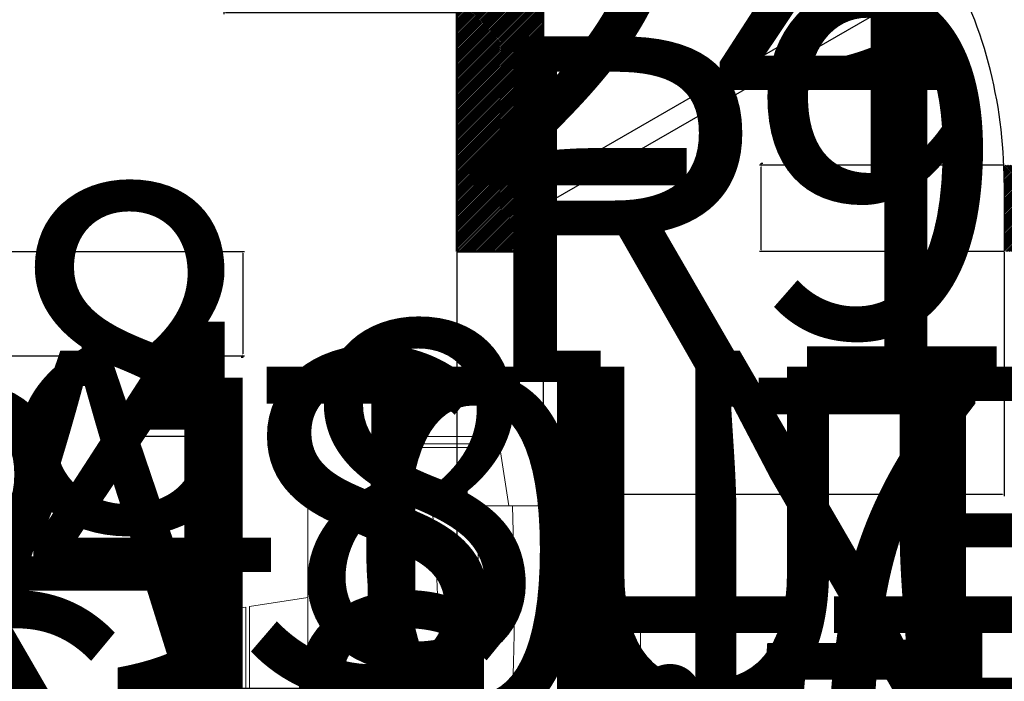
# Model space of a CAD drawing. Units: inches. Extents: x 1173 to 2157, y 515 to 1129.
# Tile 6 of 13: x 1475 to 1578, y 880 to 948. Entities that reach past the tile are written whole.
import ezdxf

# ---------------------------------------------------------------- set-up
doc = ezdxf.new("R2010")
doc.units = ezdxf.units.IN
doc.header["$MEASUREMENT"] = 0
for name, color, linetype, lineweight in [('A-ANNO-DIMS', 2, 'Continuous', 18), ('A-DOOR', 3, 'Continuous', 25), ('A-FURN', 8, 'Continuous', 18), ('A-WALL', 7, 'Continuous', 50)]:
    doc.layers.add(name, color=color, linetype=linetype, lineweight=lineweight)
doc.layers.add('A-WALL-PATT', color=22, linetype='Continuous', lineweight=13, true_color=0xca4b0c)
doc.styles.get("Standard").update_dxf_attribs({"font": 'arial.ttf'})
doc.dimstyles.get("Standard").update_dxf_attribs({"dimtxt": 36, "dimasz": 0.18, "dimexe": 0.18, "dimexo": 0.0625, "dimgap": 0.09, "dimtad": 0, "dimtih": 1, "dimtoh": 1, "dimdec": 0, "dimrnd": 72, "dimzin": 0, "dimdsep": 46, "dimlunit": 3, "dimtxsty": 'Standard', "dimcen": 2, "dimadec": 0, "dimazin": 0, "dimtfac": 1, "dimtdec": 0, "dimtofl": 0, "dimtmove": 0, "dimatfit": 3, "dimfxl": 1, "dimtolj": 1, "dimtzin": 0, "dimarcsym": 0})

# ---------------------------------------------------------------- blocks, each defined once
blk = doc.blocks.new('*U3')
for p, q in [((0, 0), (0, -6)), ((40, 0), (40, -6))]:
    blk.add_line(p, q)
blk.add_lwpolyline([(0, 0), (34.641, 20), (35.516, 18.484), (0.875, -1.516)], close=True)
blk.add_arc((0, 0), 40, 0, 30)
blk = doc.blocks.new('Dining Set - 36 x 72 in.')
for p, q in [((-22, 27.5), (-22.1562, 26.50042)), ((-22, 27.5), (-6, 27.5)), ((-5.8437, 26.49966), (-6, 27.5)), ((6, 27.5), (5.8438, 26.50042)), ((6, 27.5), (22, 27.5)), ((22.1563, 26.49966), (22, 27.5)), ((-22.2343, 26.00059), (-23.4847, 17.99762)), ((-22.2304, 26), (-5.7608, 26)), ((-5.8416, 26.5), (-22.1534, 26.5)), ((-4.5152, 17.99762), (-5.7655, 25.99926)), ((5.7657, 26.00059), (4.5153, 17.99762)), ((5.7696, 26), (22.2392, 26)), ((22.1584, 26.5), (5.8466, 26.5)), ((23.4848, 17.99762), (22.2345, 25.99926)), ((36, 18), (-36, 18)), ((-36, 18), (-36, -18)), ((36, -18), (36, 18)), ((-44.0006, 8.23428), (-35.9976, 9.48474)), ((44.0006, 8.23428), (35.9976, 9.48474)), ((-45.5, 8), (-44.5004, 8.15617)), ((-44.5, -8.15843), (-44.5, 8.15338)), ((-44, 8.23041), (-44, -8.23915)), ((44, 8.23041), (44, -8.23915)), ((44.5, -8.15843), (44.5, 8.15338)), ((45.5, 8), (44.5005, 8.15617)), ((-45.5, 8), (-45.5, -8)), ((45.5, 8), (45.5, -8)), ((-44.4997, -8.15631), (-45.5, -8)), ((44.4997, -8.15631), (45.5, -8)), ((-35.9976, -9.48476), (-43.9993, -8.2345)), ((35.9976, -9.48476), (43.9993, -8.2345)), ((-36, -18), (36, -18)), ((-22.2343, -26.0006), (-23.4847, -17.99762)), ((-4.5152, -17.99762), (-5.7655, -25.99928)), ((5.7657, -26.0006), (4.5153, -17.99762)), ((23.4848, -17.99762), (22.2345, -25.99928)), ((-22.2304, -26), (-5.7608, -26)), ((-22, -27.5), (-22.1562, -26.50044)), ((-5.8416, -26.5), (-22.1534, -26.5)), ((-5.8437, -26.49967), (-6, -27.5)), ((5.7696, -26), (22.2392, -26)), ((6, -27.5), (5.8438, -26.50044)), ((22.1584, -26.5), (5.8466, -26.5)), ((22.1563, -26.49967), (22, -27.5)), ((-22, -27.5), (-6, -27.5)), ((6, -27.5), (22, -27.5))]:
    blk.add_line(p, q)
for points in [[(-36, 15), (-31.1772, 14.97754), (-26.8079, 14.91406), (-22.8538, 14.81543), (-19.276, 14.6875), (-16.0362, 14.53613), (-13.0957, 14.36718), (-10.4159, 14.18652), (-7.9583, 14), (-5.6904, 13.81315), (-3.6035, 13.63021), (-1.6954, 13.45508), (0.0365, 13.29166), (1.5945, 13.14388), (2.9811, 13.01562), (4.1988, 12.9108), (5.25, 12.83333), (6.1393, 12.78613), (6.8802, 12.76823), (7.4883, 12.77767), (7.9792, 12.8125), (8.3685, 12.87077), (8.6719, 12.95052), (8.9049, 13.0498), (9.0833, 13.16666), (9.2205, 13.29899), (9.3216, 13.44401), (9.3895, 13.59879), (9.4271, 13.76041), (9.4373, 13.92594), (9.4232, 14.09245), (9.3875, 14.257), (9.3333, 14.41666), (9.2638, 14.56917), (9.1836, 14.71484), (9.0975, 14.85465), (9.0104, 14.98958), (8.9272, 15.1206), (8.8529, 15.2487), (8.7922, 15.37483), (8.75, 15.5), (8.7305, 15.62467), (8.7344, 15.74739), (8.7617, 15.86621), (8.8125, 15.97916), (8.8867, 16.08431), (8.9844, 16.17968), (9.1055, 16.26334), (9.25, 16.33333), (9.4189, 16.38802), (9.6172, 16.42708), (9.8506, 16.45052), (10.125, 16.45833), (10.4463, 16.45052), (10.8203, 16.42708), (11.2529, 16.38802), (11.75, 16.33333), (12.3184, 16.26318), (12.9694, 16.17838), (13.7151, 16.07991), (14.5677, 15.96875), (15.5395, 15.84586), (16.6426, 15.71224), (17.8893, 15.56884), (19.2917, 15.41666), (20.859, 15.25667), (22.5879, 15.08984), (24.4721, 14.91715), (26.5052, 14.73958), (28.6809, 14.5581), (30.9929, 14.3737), (33.4347, 14.18733), (36, 14)], [(-36, 10), (-28.9766, 10.14274), (-23.1725, 10.20442), (-18.4241, 10.19775), (-14.5677, 10.13541), (-11.4399, 10.03011), (-8.877, 9.89453), (-6.7154, 9.74137), (-4.7917, 9.58333), (-2.9698, 9.43082), (-1.2246, 9.28515), (0.4415, 9.14534), (2.026, 9.01041), (3.5266, 8.87939), (4.9408, 8.7513), (6.266, 8.62516), (7.5, 8.5), (8.6411, 8.37549), (9.6914, 8.2539), (10.6538, 8.13818), (11.5312, 8.03125), (12.3267, 7.93603), (13.043, 7.85547), (13.6831, 7.79248), (14.25, 7.75), (14.7471, 7.7303), (15.1797, 7.73307), (15.5537, 7.75732), (15.875, 7.80208), (16.1494, 7.86637), (16.3828, 7.94922), (16.5811, 8.04964), (16.75, 8.16666), (16.8944, 8.29915), (17.0143, 8.44531), (17.1089, 8.60319), (17.1771, 8.77083), (17.218, 8.94629), (17.2305, 9.1276), (17.2137, 9.31282), (17.1667, 9.5), (17.0895, 9.6875), (16.987, 9.875), (16.8649, 10.0625), (16.7292, 10.25), (16.5856, 10.4375), (16.4401, 10.625), (16.2985, 10.8125), (16.1667, 11), (16.05, 11.18733), (15.9518, 11.3737), (15.8752, 11.5581), (15.8229, 11.73958), (15.798, 11.91715), (15.8034, 12.08984), (15.842, 12.25667), (15.9167, 12.41666), (16.0295, 12.56836), (16.1784, 12.70833), (16.3605, 12.83268), (16.5729, 12.9375), (16.8127, 13.01888), (17.0768, 13.07291), (17.3625, 13.0957), (17.6667, 13.08333), (17.9894, 13.03312), (18.3418, 12.94726), (18.7382, 12.82918), (19.1927, 12.68229), (19.7195, 12.51001), (20.3327, 12.31575), (21.0465, 12.10294), (21.875, 11.875), (22.8357, 11.63354), (23.959, 11.37304), (25.2786, 11.08618), (26.8282, 10.76562), (28.6414, 10.40405), (30.752, 9.99414), (33.1936, 9.52856), (36, 9)], [(-36, 5.5), (-30.7157, 5.3348), (-26.069, 5.20963), (-21.9946, 5.11767), (-18.4271, 5.05208), (-15.3009, 5.00602), (-12.5508, 4.97265), (-10.1112, 4.94515), (-7.9167, 4.91666), (-5.909, 4.88167), (-4.0586, 4.83984), (-2.3429, 4.79215), (-0.7396, 4.73958), (0.7739, 4.6831), (2.22, 4.6237), (3.6213, 4.56233), (5, 4.5), (6.373, 4.43782), (7.7344, 4.3776), (9.0723, 4.32129), (10.375, 4.27083), (11.6309, 4.22819), (12.8281, 4.19531), (13.9551, 4.17415), (15, 4.16666), (15.954, 4.17448), (16.819, 4.19791), (17.6001, 4.23698), (18.3021, 4.29166), (18.9299, 4.36198), (19.4883, 4.44791), (19.9823, 4.54948), (20.4167, 4.66666), (20.7969, 4.79899), (21.1302, 4.94401), (21.4245, 5.09879), (21.6875, 5.26041), (21.9271, 5.42594), (22.1511, 5.59245), (22.3672, 5.757), (22.5834, 5.91666), (22.8065, 6.06868), (23.0404, 6.21093), (23.2879, 6.34147), (23.5521, 6.45833), (23.8358, 6.55957), (24.142, 6.64323), (24.4735, 6.70735), (24.8334, 6.75), (25.2235, 6.76969), (25.642, 6.76692), (26.0858, 6.74267), (26.5521, 6.69791), (27.0379, 6.63362), (27.5404, 6.55078), (28.0565, 6.45036), (28.5834, 6.33333), (29.1242, 6.19987), (29.7071, 6.04687), (30.3661, 5.87044), (31.1354, 5.66666), (32.0493, 5.43164), (33.142, 5.16146), (34.4475, 4.85221), (36, 4.5)], [(-36, -1), (-30.7915, -0.6591), (-26.0195, -0.38216), (-21.6519, -0.16284), (-17.6563, 0.00521), (-14.0005, 0.12833), (-10.6523, 0.21289), (-7.5796, 0.26522), (-4.75, 0.29166), (-2.134, 0.29793), (0.2878, 0.28711), (2.5317, 0.26163), (4.6146, 0.22396), (6.5529, 0.17651), (8.3633, 0.12174), (10.0623, 0.06209), (11.6667, 0), (13.1899, -0.06201), (14.6341, -0.1211), (15.9982, -0.17432), (17.2813, -0.21875), (18.4823, -0.25147), (19.6003, -0.26953), (20.6343, -0.27002), (21.5834, -0.25), (22.4481, -0.20768), (23.2357, -0.14584), (23.9549, -0.06836), (24.6146, 0.02083), (25.2235, 0.11784), (25.7904, 0.21875), (26.3241, 0.31966), (26.8334, 0.41666), (27.3265, 0.50618), (27.8099, 0.58593), (28.2894, 0.65397), (28.7709, 0.70833), (29.2601, 0.74707), (29.763, 0.76823), (30.2855, 0.76985), (30.8334, 0.75), (31.4088, 0.70784), (31.9994, 0.64713), (32.589, 0.57275), (33.1615, 0.48958), (33.7008, 0.4025), (34.1908, 0.3164), (34.6153, 0.23616), (34.9584, 0.16666), (35.2099, 0.11165), (35.3848, 0.07031), (35.504, 0.04069), (35.5886, 0.02083), (35.6594, 0.00879), (35.7377, 0.0026), (35.8442, 0.00032), (36, 0)], [(-36, -6.5), (-27.1843, -6.31267), (-20.084, -6.1263), (-14.469, -5.9419), (-10.1094, -5.76042), (-6.7752, -5.58285), (-4.2363, -5.41016), (-2.2629, -5.24333), (-0.625, -5.08334), (0.8708, -4.93099), (2.2715, -4.78646), (3.5872, -4.64974), (4.8281, -4.52084), (6.0046, -4.39974), (7.127, -4.28646), (8.2053, -4.18099), (9.25, -4.08334), (10.2705, -3.99382), (11.2734, -3.91407), (12.2647, -3.84603), (13.25, -3.79167), (14.2354, -3.75293), (15.2266, -3.73177), (16.2295, -3.73015), (17.25, -3.75), (18.2912, -3.79248), (19.3451, -3.85547), (20.4009, -3.93604), (21.4479, -4.03125), (22.4754, -4.13819), (23.4727, -4.25391), (24.4289, -4.37549), (25.3334, -4.5), (26.1785, -4.62492), (26.9694, -4.74935), (27.7145, -4.87281), (28.4219, -4.99479), (29.1, -5.11483), (29.7572, -5.23242), (30.4016, -5.34709), (31.0417, -5.45834), (31.6837, -5.56437), (32.3262, -5.65821), (32.9658, -5.73153), (33.599, -5.77604), (34.2224, -5.78345), (34.8327, -5.74545), (35.4264, -5.65373), (36, -5.5)], [(-36, -10), (-26.4022, -9.81299), (-18.4675, -9.62891), (-11.9839, -9.45069), (-6.7396, -9.28125), (-2.5226, -9.12354), (0.8789, -8.98047), (3.6769, -8.85498), (6.0833, -8.75), (8.2767, -8.66765), (10.3021, -8.60677), (12.1712, -8.56543), (13.8958, -8.54167), (15.4876, -8.53353), (16.9583, -8.53907), (18.3197, -8.55632), (19.5834, -8.58334), (20.7616, -8.61841), (21.8685, -8.66081), (22.9188, -8.71004), (23.9271, -8.76563), (24.9081, -8.82707), (25.8763, -8.89388), (26.8465, -8.96558), (27.8334, -9.04167), (28.8474, -9.12118), (29.8828, -9.20117), (30.93, -9.27824), (31.9792, -9.34896), (33.0205, -9.40991), (34.0443, -9.45768), (35.0407, -9.48885), (36, -9.5)], [(-36, -14.5), (-30.0881, -14.33513), (-25.0332, -14.21224), (-20.7312, -14.12647), (-17.0781, -14.07292), (-13.97, -14.04671), (-11.3027, -14.04297), (-8.9724, -14.05681), (-6.875, -14.08334), (-4.9224, -14.11833), (-3.0905, -14.16016), (-1.3709, -14.20785), (0.2448, -14.26042), (1.7647, -14.3169), (3.1973, -14.3763), (4.5507, -14.43767), (5.8333, -14.5), (7.0554, -14.5621), (8.235, -14.62175), (9.3922, -14.67652), (10.5469, -14.72396), (11.7192, -14.76164), (12.929, -14.78711), (14.1965, -14.79794), (15.5417, -14.79167), (16.9933, -14.76424), (18.6152, -14.70508), (20.4804, -14.60197), (22.6615, -14.44271), (25.2312, -14.21509), (28.2624, -13.9069), (31.8277, -13.50594), (36, -13)]]:
    blk.add_lwpolyline(points)
blk = doc.blocks.new('*D36')
at = {"layer": 'A-ANNO-DIMS', "color": 0, "lineweight": -2, "transparency": 16777216}
for p, q in [((1497.87, 905.02), (1487.37, 905.02)), ((1487.55, 904.84), (1487.55, 889.09)), ((1487.55, 835.93), (1487.55, 851.68)), ((1497.87, 835.75), (1487.37, 835.75))]:
    blk.add_line(p, q, dxfattribs=at)
at = {"layer": 'A-ANNO-DIMS', "color": 0, "transparency": 16777216}
for points in [[(1487.52, 904.84), (1487.58, 904.84), (1487.55, 905.02)], [(1487.52, 835.93), (1487.58, 835.93), (1487.55, 835.75)]]:
    blk.add_solid(points, dxfattribs=at)
at = {"layer": 'Defpoints', "color": 0, "transparency": 16777216}
for p in [(1497.94, 905.02), (1487.55, 835.75), (1497.94, 835.75)]:
    blk.add_point(p, dxfattribs=at)
at = {"layer": 'A-ANNO-DIMS', "color": 0, "transparency": 16777216, "insert": (1487.55, 870.38), "char_height": 36, "attachment_point": 5}
blk.add_mtext('\\A1;DINING SET 69', dxfattribs=at)
blk = doc.blocks.new('*D38')
at = {"layer": 'A-ANNO-DIMS', "color": 0, "lineweight": -2, "transparency": 16777216}
for p, q in [((1471.69, 862.7), (1478.04, 862.7)), ((1477.86, 862.52), (1477.86, 860.65)), ((1477.86, 821.35), (1477.86, 823.22)), ((1471.69, 821.17), (1478.04, 821.17))]:
    blk.add_line(p, q, dxfattribs=at)
at = {"layer": 'A-ANNO-DIMS', "color": 0, "transparency": 16777216}
for points in [[(1477.83, 862.52), (1477.89, 862.52), (1477.86, 862.7)], [(1477.83, 821.35), (1477.89, 821.35), (1477.86, 821.17)]]:
    blk.add_solid(points, dxfattribs=at)
at = {"layer": 'Defpoints', "color": 0, "transparency": 16777216}
for p in [(1471.63, 862.7), (1477.86, 862.7), (1471.63, 821.17)]:
    blk.add_point(p, dxfattribs=at)
at = {"layer": 'A-ANNO-DIMS', "color": 0, "transparency": 16777216, "insert": (1477.86, 841.93), "char_height": 36, "attachment_point": 5}
blk.add_mtext('\\A1;COFFEE TABLE 42', dxfattribs=at)
blk = doc.blocks.new('*D40')
at = {"layer": 'A-ANNO-DIMS', "color": 0, "lineweight": -2, "transparency": 16777216}
for p, q in [((1422.73, 872.86), (1431.84, 872.86)), ((1431.66, 872.68), (1431.66, 861.58)), ((1431.66, 813.04), (1431.66, 824.15)), ((1422.73, 812.86), (1431.84, 812.86))]:
    blk.add_line(p, q, dxfattribs=at)
at = {"layer": 'A-ANNO-DIMS', "color": 0, "transparency": 16777216}
for points in [[(1431.63, 872.68), (1431.69, 872.68), (1431.66, 872.86)], [(1431.63, 813.04), (1431.69, 813.04), (1431.66, 812.86)]]:
    blk.add_solid(points, dxfattribs=at)
at = {"layer": 'Defpoints', "color": 0, "transparency": 16777216}
for p in [(1422.66, 872.86), (1431.66, 872.86), (1422.66, 812.86)]:
    blk.add_point(p, dxfattribs=at)
at = {"layer": 'A-ANNO-DIMS', "color": 0, "transparency": 16777216, "insert": (1431.66, 842.86), "char_height": 36, "attachment_point": 5}
blk.add_mtext('\\A1;LOVESEAT 60', dxfattribs=at)
blk = doc.blocks.new('*D46')
at = {"layer": 'A-ANNO-DIMS', "color": 0, "lineweight": -2, "transparency": 16777216}
for p, q in [((1646.37, 911.98), (1645.86, 896.32)), ((1648.72, 912.09), (1646.2, 912.17)), ((1645.85, 895.96), (1645.67, 895.96)), ((1648.2, 896.07), (1645.68, 896.15)), ((1645.86, 896.14), (1645.85, 895.96))]:
    blk.add_line(p, q, dxfattribs=at)
at = {"layer": 'A-ANNO-DIMS', "color": 0, "transparency": 16777216}
for points in [[(1646.34, 911.99), (1646.4, 911.98), (1646.38, 912.16)], [(1645.83, 896.32), (1645.89, 896.32), (1645.86, 896.14)]]:
    blk.add_solid(points, dxfattribs=at)
at = {"layer": 'Defpoints', "color": 0, "transparency": 16777216}
for p in [(1648.78, 912.09), (1645.86, 896.14), (1648.26, 896.06)]:
    blk.add_point(p, dxfattribs=at)
at = {"layer": 'A-ANNO-DIMS', "color": 0, "transparency": 16777216, "insert": (1538.16, 895.96), "char_height": 36, "attachment_point": 5}
blk.add_mtext('\\A1;BASIN 16', dxfattribs=at)
blk = doc.blocks.new('*D48')
at = {"layer": 'A-ANNO-DIMS', "color": 0, "lineweight": -2, "transparency": 16777216}
for p, q in [((1592.53, 826.46), (1592.35, 826.47)), ((1592.38, 821.85), (1592.54, 826.64)), ((1623.53, 825.46), (1592.71, 826.46)), ((1623.56, 820.84), (1623.71, 825.64))]:
    blk.add_line(p, q, dxfattribs=at)
at = {"layer": 'A-ANNO-DIMS', "color": 0, "transparency": 16777216}
for points in [[(1592.71, 826.49), (1592.71, 826.43), (1592.53, 826.46)], [(1623.53, 825.49), (1623.53, 825.43), (1623.71, 825.46)]]:
    blk.add_solid(points, dxfattribs=at)
at = {"layer": 'Defpoints', "color": 0, "transparency": 16777216}
for p in [(1592.53, 826.46), (1592.38, 821.79), (1623.56, 820.78)]:
    blk.add_point(p, dxfattribs=at)
at = {"layer": 'A-ANNO-DIMS', "color": 0, "transparency": 16777216, "insert": (1488.3, 826.47), "char_height": 36, "attachment_point": 5}
blk.add_mtext('\\A1;BASIN 31', dxfattribs=at)
blk = doc.blocks.new('*D50')
at = {"layer": 'A-ANNO-DIMS', "color": 0, "lineweight": -2, "transparency": 16777216}
for p, q in [((1603.33, 798.21), (1603.33, 796.59)), ((1613.33, 798.21), (1613.33, 796.59)), ((1603.33, 796.77), (1603.15, 796.77)), ((1613.15, 796.77), (1603.51, 796.77))]:
    blk.add_line(p, q, dxfattribs=at)
at = {"layer": 'A-ANNO-DIMS', "color": 0, "transparency": 16777216}
for points in [[(1603.51, 796.8), (1603.51, 796.74), (1603.33, 796.77)], [(1613.15, 796.8), (1613.15, 796.74), (1613.33, 796.77)]]:
    blk.add_solid(points, dxfattribs=at)
at = {"layer": 'Defpoints', "color": 0, "transparency": 16777216}
for p in [(1603.33, 798.27), (1613.33, 798.27), (1603.33, 796.77)]:
    blk.add_point(p, dxfattribs=at)
at = {"layer": 'A-ANNO-DIMS', "color": 0, "transparency": 16777216, "insert": (1377.9, 796.77), "char_height": 36, "attachment_point": 5}
blk.add_mtext('\\A1;BASIN TAP 10 TYP.', dxfattribs=at)
blk = doc.blocks.new('*D52')
at = {"layer": 'A-ANNO-DIMS', "color": 0, "lineweight": -2, "transparency": 16777216}
for p, q in [((1589.6, 924.28), (1580.48, 924.28)), ((1580.66, 924.1), (1580.66, 912.75)), ((1580.66, 864.46), (1580.66, 875.81)), ((1589.6, 864.28), (1580.48, 864.28))]:
    blk.add_line(p, q, dxfattribs=at)
at = {"layer": 'A-ANNO-DIMS', "color": 0, "transparency": 16777216}
for points in [[(1580.63, 924.1), (1580.69, 924.1), (1580.66, 924.28)], [(1580.63, 864.46), (1580.69, 864.46), (1580.66, 864.28)]]:
    blk.add_solid(points, dxfattribs=at)
at = {"layer": 'Defpoints', "color": 0, "transparency": 16777216}
for p in [(1580.66, 924.28), (1589.66, 924.28), (1589.66, 864.28)]:
    blk.add_point(p, dxfattribs=at)
at = {"layer": 'A-ANNO-DIMS', "color": 0, "transparency": 16777216, "insert": (1580.66, 894.28), "char_height": 36, "attachment_point": 5}
blk.add_mtext('\\A1;TUB 60', dxfattribs=at)
blk = doc.blocks.new('*D54')
at = {"layer": 'A-ANNO-DIMS', "color": 0, "lineweight": -2, "transparency": 16777216}
for p, q in [((1496.35, 1005.18), (1488.93, 1005.18)), ((1489.11, 1005), (1489.11, 999.54)), ((1489.11, 956.65), (1489.11, 962.11)), ((1496.35, 956.47), (1488.93, 956.47))]:
    blk.add_line(p, q, dxfattribs=at)
at = {"layer": 'A-ANNO-DIMS', "color": 0, "transparency": 16777216}
for points in [[(1489.08, 1005), (1489.14, 1005), (1489.11, 1005.18)], [(1489.08, 956.65), (1489.14, 956.65), (1489.11, 956.47)]]:
    blk.add_solid(points, dxfattribs=at)
at = {"layer": 'Defpoints', "color": 0, "transparency": 16777216}
for p in [(1496.42, 1005.18), (1489.11, 956.47), (1496.42, 956.47)]:
    blk.add_point(p, dxfattribs=at)
at = {"layer": 'A-ANNO-DIMS', "color": 0, "transparency": 16777216, "insert": (1489.11, 980.83), "char_height": 36, "attachment_point": 5}
blk.add_mtext('\\A1;WORK TABLE 49', dxfattribs=at)
blk = doc.blocks.new('*D55')
at = {"layer": 'A-ANNO-DIMS', "color": 0, "lineweight": -2, "transparency": 16777216}
for p, q in [((1496.42, 956.41), (1496.42, 948.98)), ((1520.77, 956.41), (1520.77, 948.98)), ((1496.6, 949.16), (1520.59, 949.16)), ((1520.77, 949.16), (1520.95, 949.16))]:
    blk.add_line(p, q, dxfattribs=at)
at = {"layer": 'A-ANNO-DIMS', "color": 0, "transparency": 16777216}
for points in [[(1496.6, 949.19), (1496.6, 949.13), (1496.42, 949.16)], [(1520.59, 949.19), (1520.59, 949.13), (1520.77, 949.16)]]:
    blk.add_solid(points, dxfattribs=at)
at = {"layer": 'Defpoints', "color": 0, "transparency": 16777216}
for p in [(1496.42, 956.47), (1520.77, 956.47), (1520.77, 949.16)]:
    blk.add_point(p, dxfattribs=at)
at = {"layer": 'A-ANNO-DIMS', "color": 0, "transparency": 16777216, "insert": (1547.06, 949.16), "char_height": 36, "attachment_point": 5}
blk.add_mtext('\\A1;24', dxfattribs=at)
blk = doc.blocks.new('*D56')
at = {"layer": 'A-ANNO-DIMS', "color": 0, "lineweight": -2, "transparency": 16777216}
for p, q in [((1426.92, 1014.79), (1433.2, 1014.79)), ((1433.02, 1014.61), (1433.02, 1012.98)), ((1433.02, 973.94), (1433.02, 975.57)), ((1426.92, 973.76), (1433.2, 973.76))]:
    blk.add_line(p, q, dxfattribs=at)
at = {"layer": 'A-ANNO-DIMS', "color": 0, "transparency": 16777216}
for points in [[(1432.99, 1014.61), (1433.05, 1014.61), (1433.02, 1014.79)], [(1432.99, 973.94), (1433.05, 973.94), (1433.02, 973.76)]]:
    blk.add_solid(points, dxfattribs=at)
at = {"layer": 'Defpoints', "color": 0, "transparency": 16777216}
for p in [(1426.86, 1014.79), (1433.02, 1014.79), (1426.86, 973.76)]:
    blk.add_point(p, dxfattribs=at)
at = {"layer": 'A-ANNO-DIMS', "color": 0, "transparency": 16777216, "insert": (1433.02, 994.27), "char_height": 36, "attachment_point": 5}
blk.add_mtext('\\A1;RANGE 41', dxfattribs=at)
blk = doc.blocks.new('*D60')
at = {"layer": 'A-ANNO-DIMS', "color": 0, "lineweight": -2, "transparency": 16777216}
for p, q in [((1390.73, 971.62), (1390.73, 971.8)), ((1390.73, 971.8), (1390.91, 971.8)), ((1396.06, 971.62), (1390.55, 971.62)), ((1390.73, 935.8), (1390.73, 971.44)), ((1396.06, 935.62), (1390.55, 935.62))]:
    blk.add_line(p, q, dxfattribs=at)
at = {"layer": 'A-ANNO-DIMS', "color": 0, "transparency": 16777216}
for points in [[(1390.7, 971.44), (1390.76, 971.44), (1390.73, 971.62)], [(1390.7, 935.8), (1390.76, 935.8), (1390.73, 935.62)]]:
    blk.add_solid(points, dxfattribs=at)
at = {"layer": 'Defpoints', "color": 0, "transparency": 16777216}
for p in [(1390.73, 971.62), (1396.13, 971.62), (1396.13, 935.62)]:
    blk.add_point(p, dxfattribs=at)
at = {"layer": 'A-ANNO-DIMS', "color": 0, "transparency": 16777216, "insert": (1517.73, 971.8), "char_height": 36, "attachment_point": 5}
blk.add_mtext('\\A1;FRIDGE 36', dxfattribs=at)
blk = doc.blocks.new('*D69')
at = {"layer": 'A-ANNO-DIMS', "color": 0, "lineweight": -2, "transparency": 16777216}
for p, q in [((1472.66, 924.22), (1472.66, 538.8)), ((1520.66, 924.22), (1520.66, 538.8)), ((1472.84, 538.98), (1520.48, 538.98)), ((1520.66, 538.98), (1520.84, 538.98))]:
    blk.add_line(p, q, dxfattribs=at)
at = {"layer": 'A-ANNO-DIMS', "color": 0, "transparency": 16777216}
for points in [[(1472.84, 539.01), (1472.84, 538.95), (1472.66, 538.98)], [(1520.48, 539.01), (1520.48, 538.95), (1520.66, 538.98)]]:
    blk.add_solid(points, dxfattribs=at)
at = {"layer": 'Defpoints', "color": 0, "transparency": 16777216}
for p in [(1472.66, 924.28), (1520.66, 924.28), (1520.66, 538.98)]:
    blk.add_point(p, dxfattribs=at)
at = {"layer": 'A-ANNO-DIMS', "color": 0, "transparency": 16777216, "insert": (1547.48, 538.98), "char_height": 36, "attachment_point": 5}
blk.add_mtext('\\A1;48', dxfattribs=at)
blk = doc.blocks.new('*D87')
at = {"layer": 'A-ANNO-DIMS', "color": 0, "lineweight": -2, "transparency": 16777216}
for p, q in [((1529.66, 924.22), (1529.66, 898.8)), ((1577.66, 924.22), (1577.66, 898.8)), ((1529.66, 898.98), (1529.48, 898.98)), ((1577.48, 898.98), (1529.84, 898.98))]:
    blk.add_line(p, q, dxfattribs=at)
at = {"layer": 'A-ANNO-DIMS', "color": 0, "transparency": 16777216}
for points in [[(1529.84, 899.01), (1529.84, 898.95), (1529.66, 898.98)], [(1577.48, 899.01), (1577.48, 898.95), (1577.66, 898.98)]]:
    blk.add_solid(points, dxfattribs=at)
at = {"layer": 'Defpoints', "color": 0, "transparency": 16777216}
for p in [(1529.66, 924.28), (1577.66, 924.28), (1529.66, 898.98)]:
    blk.add_point(p, dxfattribs=at)
at = {"layer": 'A-ANNO-DIMS', "color": 0, "transparency": 16777216, "insert": (1502.85, 898.98), "char_height": 36, "attachment_point": 5}
blk.add_mtext('\\A1;48', dxfattribs=at)
blk = doc.blocks.new('*D93')
at = {"layer": 'A-ANNO-DIMS', "color": 0, "lineweight": -2, "transparency": 16777216}
for p, q in [((1473.15, 924.28), (1498.57, 924.28)), ((1498.39, 924.1), (1498.39, 913.61)), ((1473.15, 913.43), (1498.57, 913.43)), ((1498.39, 913.25), (1498.21, 913.25)), ((1498.39, 913.43), (1498.39, 913.25))]:
    blk.add_line(p, q, dxfattribs=at)
at = {"layer": 'A-ANNO-DIMS', "color": 0, "transparency": 16777216}
for points in [[(1498.36, 924.1), (1498.42, 924.1), (1498.39, 924.28)], [(1498.36, 913.61), (1498.42, 913.61), (1498.39, 913.43)]]:
    blk.add_solid(points, dxfattribs=at)
at = {"layer": 'Defpoints', "color": 0, "transparency": 16777216}
for p in [(1473.08, 924.28), (1473.08, 913.43), (1498.39, 913.43)]:
    blk.add_point(p, dxfattribs=at)
at = {"layer": 'A-ANNO-DIMS', "color": 0, "transparency": 16777216, "insert": (1425.05, 913.25), "char_height": 36, "attachment_point": 5}
blk.add_mtext('\\A1;10.848', dxfattribs=at)
blk = doc.blocks.new('*D94')
at = {"layer": 'A-ANNO-DIMS', "color": 0, "lineweight": -2, "transparency": 16777216}
for p, q in [((1577.6, 933.28), (1552.18, 933.28)), ((1552.36, 933.28), (1552.36, 933.46)), ((1552.36, 933.46), (1552.54, 933.46)), ((1552.36, 924.46), (1552.36, 933.1)), ((1577.6, 924.28), (1552.18, 924.28))]:
    blk.add_line(p, q, dxfattribs=at)
at = {"layer": 'A-ANNO-DIMS', "color": 0, "transparency": 16777216}
for points in [[(1552.33, 933.1), (1552.39, 933.1), (1552.36, 933.28)], [(1552.33, 924.46), (1552.39, 924.46), (1552.36, 924.28)]]:
    blk.add_solid(points, dxfattribs=at)
at = {"layer": 'Defpoints', "color": 0, "transparency": 16777216}
for p in [(1552.36, 933.28), (1577.66, 933.28), (1577.66, 924.28)]:
    blk.add_point(p, dxfattribs=at)
at = {"layer": 'A-ANNO-DIMS', "color": 0, "transparency": 16777216, "insert": (1564.47, 933.46), "char_height": 36, "attachment_point": 5}
blk.add_mtext('\\A1;9', dxfattribs=at)
blk = doc.blocks.new('*D107')
at = {"layer": 'A-ANNO-DIMS', "color": 0, "lineweight": -2, "transparency": 16777216}
for p, q in [((1607.48, 928.68), (1607.66, 928.68)), ((1607.66, 928.68), (1607.66, 920.46)), ((1607.66, 904.28), (1607.66, 908.28)), ((1605.66, 906.28), (1609.66, 906.28))]:
    blk.add_line(p, q, dxfattribs=at)
at = {"layer": 'A-ANNO-DIMS', "color": 0, "transparency": 16777216}
blk.add_solid([(1607.69, 920.46), (1607.63, 920.46), (1607.66, 920.28)], dxfattribs=at)
at = {"layer": 'Defpoints', "color": 0, "transparency": 16777216}
for p in [(1607.66, 920.28), (1607.66, 906.28)]:
    blk.add_point(p, dxfattribs=at)
at = {"layer": 'A-ANNO-DIMS', "color": 0, "transparency": 16777216, "insert": (1564.46, 928.68), "char_height": 36, "attachment_point": 5}
blk.add_mtext('\\A1;R14', dxfattribs=at)
blk = doc.blocks.new('*D108')
at = {"layer": 'A-ANNO-DIMS', "color": 0, "lineweight": -2, "transparency": 16777216}
for p, q in [((1641.43, 881.4), (1641.43, 885.4)), ((1639.43, 883.4), (1643.43, 883.4)), ((1636.72, 865.51), (1638.44, 872.04)), ((1636.54, 865.51), (1636.72, 865.51))]:
    blk.add_line(p, q, dxfattribs=at)
at = {"layer": 'A-ANNO-DIMS', "color": 0, "transparency": 16777216}
blk.add_solid([(1638.41, 872.05), (1638.47, 872.04), (1638.49, 872.22)], dxfattribs=at)
at = {"layer": 'Defpoints', "color": 0, "transparency": 16777216}
for p in [(1641.43, 883.4), (1638.49, 872.22)]:
    blk.add_point(p, dxfattribs=at)
at = {"layer": 'A-ANNO-DIMS', "color": 0, "transparency": 16777216, "insert": (1505.59, 865.51), "char_height": 36, "attachment_point": 5}
blk.add_mtext('\\A1;2X R11.564', dxfattribs=at)
blk = doc.blocks.new('*D109')
at = {"layer": 'A-ANNO-DIMS', "color": 0, "lineweight": -2, "transparency": 16777216}
for p, q in [((1638.72, 893.14), (1638.9, 893.14)), ((1638.9, 893.14), (1639.74, 886.91)), ((1641.2, 874.07), (1641.2, 878.07)), ((1639.2, 876.07), (1643.2, 876.07))]:
    blk.add_line(p, q, dxfattribs=at)
at = {"layer": 'A-ANNO-DIMS', "color": 0, "transparency": 16777216}
blk.add_solid([(1639.77, 886.92), (1639.71, 886.91), (1639.77, 886.74)], dxfattribs=at)
at = {"layer": 'Defpoints', "color": 0, "transparency": 16777216}
for p in [(1639.77, 886.74), (1641.2, 876.07)]:
    blk.add_point(p, dxfattribs=at)
at = {"layer": 'A-ANNO-DIMS', "color": 0, "transparency": 16777216, "insert": (1507.71, 893.14), "char_height": 36, "attachment_point": 5}
blk.add_mtext('\\A1;2X R10.766', dxfattribs=at)

msp = doc.modelspace()

# ---------------------------------------------------------------- hatches: boundary and pattern name
at = {"layer": 'A-WALL-PATT'}
h = msp.add_hatch(dxfattribs=at)
h.set_pattern_fill('ANSI31', color=256)
h.paths.add_polyline_path([(1388.6635, 933.2805), (1388.6635, 1044.2805), (1413.7618, 1044.2805), (1413.7618, 1053.2805), (1379.6635, 1053.2805), (1379.6635, 894.1606), (1388.6635, 894.1606), (1388.6635, 924.2805), (1472.6635, 924.2805), (1472.6635, 933.2805)])
h.paths.add_polyline_path([(1520.6635, 1044.2805), (1520.6635, 1014.7866), (1520.6635, 1005.1794), (1520.7714, 1005.1794), (1520.7714, 956.4707), (1520.6635, 924.2805), (1529.6635, 924.2805), (1529.6635, 931.4788), (1529.6635, 1044.2805), (1530.8474, 1044.2805), (1570.9543, 1044.2805), (1570.9543, 1053.2805), (1461.7618, 1053.2805), (1461.7618, 1044.2805)])
h.paths.add_polyline_path([(1618.9543, 1053.2805), (1618.9543, 1044.2805), (1661.6635, 1044.2805), (1661.6635, 1043.7367), (1661.6635, 1032.8874), (1670.6635, 1032.8874), (1670.6635, 1053.2805)])
h.paths.add_polyline_path([(1661.6635, 933.2805), (1661.6635, 927.8377), (1661.6635, 924.2805), (1661.6635, 918.9156), (1670.6635, 918.9156), (1670.6635, 984.8874), (1661.6635, 984.8874), (1661.6635, 978.3712)])
h.paths.add_polyline_path([(1670.6635, 894.9156), (1661.6635, 894.9156), (1661.6635, 890.0349), (1661.9328, 890.0349), (1661.9328, 870.079), (1661.6635, 864.2805), (1589.6635, 864.2805), (1589.6635, 924.2805), (1625.553, 924.2805, -0.02455299), (1625.3782, 927.8377), (1625.3782, 933.2805), (1577.6635, 933.2805), (1577.6635, 924.2805), (1580.6635, 924.2805), (1580.6635, 855.2805), (1586.1062, 855.2805), (1589.6635, 855.2805), (1661.6635, 855.2805), (1661.6635, 826.5597), (1670.6635, 826.5597)])
h.paths.add_polyline_path([(1670.6635, 802.5597), (1661.6635, 802.5597), (1661.6635, 795.2805), (1589.6635, 795.2805), (1589.6635, 819.17, -0.02455299), (1586.1062, 818.9952), (1580.6635, 818.9952), (1580.6635, 795.2805), (1577.6635, 795.2805), (1577.6635, 786.2805), (1661.6635, 786.2805), (1661.6635, 778.5597), (1661.6635, 742.6973), (1670.6635, 742.6973)])
h.paths.add_polyline_path([(1661.6635, 654.2805), (1625.1498, 654.2805), (1625.1498, 645.2805), (1661.3656, 645.2805), (1661.6635, 645.2805), (1661.6635, 573.2805), (1520.6635, 573.2805), (1520.6635, 564.2805), (1670.6635, 564.2805), (1670.6635, 694.6973), (1661.6635, 694.6973)])
h.paths.add_polyline_path([(1529.4367, 733.4702, -0.06854064), (1529.6635, 734.2623), (1529.6635, 795.2805), (1520.6635, 795.2805), (1520.6635, 645.2805), (1577.1498, 645.2805), (1577.1498, 654.2805), (1529.6635, 654.2805), (1529.6635, 686.5626, -0.06854064), (1529.4367, 687.3547)])
h.paths.add_polyline_path([(1379.6635, 711.2805), (1388.6635, 711.2805), (1458.7214, 711.2805), (1458.7214, 720.2805), (1410.7214, 720.2805), (1388.6635, 720.2805), (1388.6635, 745.0427), (1379.6635, 745.0427)])
h.paths.add_polyline_path([(1388.6635, 846.1606), (1379.6635, 846.1606), (1379.6635, 793.0427), (1388.6635, 793.0427)])

# ---------------------------------------------------------------- linework, layer by layer
at = {"layer": 'A-WALL'}
for p, q in [((1520.6635, 924.2805), (1520.6635, 1044.2805)), ((1529.6635, 924.2805), (1529.6635, 1044.2805)), ((1529.6635, 924.2805), (1529.6635, 1044.2805)), ((1529.6635, 924.2805), (1520.6635, 924.2805))]:
    msp.add_line(p, q, dxfattribs=at)

# ---------------------------------------------------------------- block references
at = {"layer": 'A-DOOR', "xscale": 1.199708577982686, "yscale": 1.199708577982686, "zscale": 1.199708577982686}
msp.add_blockref('*U3', (1529.6635, 931.4788), dxfattribs=at)
at = {"layer": 'A-FURN', "xscale": 0.7611912225144155, "yscale": 0.7611912225144155, "zscale": 0.7611912225144155, "rotation": 270}
msp.add_blockref('Dining Set - 36 x 72 in.', (1518.8694, 870.3828), dxfattribs=at)

# ---------------------------------------------------------------- dimensions: what is measured, and where the dimension line sits
at = {"layer": 'A-ANNO-DIMS'}
for base, p1, p2, angle, text, picture, middle in [((1489.1107, 956.4707), (1496.4171, 1005.1794), (1496.4171, 956.4707), 270, 'WORK TABLE <>', '*D54', (1489.1107, 980.8251)), ((1433.0151, 1014.7866), (1426.8605, 973.7559), (1426.8605, 1014.7866), 90, 'RANGE <>', '*D56', (1433.0151, 994.2712)), ((1390.7251, 971.618), (1396.1251, 935.618), (1396.1251, 971.618), 90, 'FRIDGE <>', '*D60', (1517.7318, 971.798)), ((1487.5464, 835.7486), (1497.9367, 905.017), (1497.9367, 835.7486), 270, 'DINING SET <>', '*D36', (1487.5464, 870.3828)), ((1645.8589, 896.1412), (1648.7786, 912.0868), (1648.2623, 896.0638), 268.15447, 'BASIN <>', '*D46', (1538.1601, 895.9613)), ((1580.6635, 924.2805), (1589.6635, 864.2805), (1589.6635, 924.2805), 90, 'TUB <>', '*D52', (1580.6635, 894.2805)), ((1477.8589, 862.6955), (1471.63, 821.1697), (1471.63, 862.6955), 90, 'COFFEE TABLE <>', '*D38', (1477.8589, 841.9326)), ((1603.3335, 796.7679), (1613.3335, 798.2679), (1603.3335, 798.2679), 180, 'BASIN TAP <> TYP.', '*D50', (1377.9039, 796.7679)), ((1431.6634, 872.8622), (1422.6634, 812.8621), (1422.6634, 872.8622), 90, 'LOVESEAT <>', '*D40', (1431.6634, 842.8622)), ((1592.531, 826.4624), (1623.5567, 820.7814), (1592.3803, 821.786), 178.15447, 'BASIN <>', '*D48', (1488.3007, 826.4682))]:
    dim = msp.add_linear_dim(base=base, p1=p1, p2=p2, angle=angle, text=text, dimstyle='Standard', override={"dimdec": 0, "dimlfac": 1, "dimrnd": 0, "dimzin": 0, "dimdsep": 46, "dimlunit": 2}, dxfattribs=at)
    dim.commit()
    dim.dimension.update_dxf_attribs({"geometry": picture, "text_midpoint": middle})
for base, p1, p2, picture, middle in [((1520.7714, 949.1644), (1496.4171, 956.4707), (1520.7714, 956.4707), '*D55', (1547.0592, 949.1644)), ((1520.6635, 538.978), (1472.6635, 924.2805), (1520.6635, 924.2805), '*D69', (1547.4792, 538.978))]:
    dim = msp.add_linear_dim(base=base, p1=p1, p2=p2, dimstyle='Standard', override={"dimdec": 0, "dimlfac": 1, "dimrnd": 0, "dimzin": 0, "dimdsep": 46, "dimlunit": 2}, dxfattribs=at)
    dim.commit()
    dim.dimension.update_dxf_attribs({"geometry": picture, "text_midpoint": middle})
for base, p1, p2, angle, override, picture, middle in [((1552.361, 933.2805), (1577.6635, 924.2805), (1577.6635, 933.2805), 90, {"dimdec": 0, "dimlfac": 1, "dimrnd": 0, "dimzin": 0, "dimdsep": 46, "dimlunit": 2}, '*D94', (1564.4672, 933.4605)), ((1498.3865, 913.4324), (1473.084, 924.2805), (1473.084, 913.4324), 270, {"dimdec": 3, "dimlfac": 1, "dimrnd": 0, "dimzin": 0, "dimdsep": 46, "dimlunit": 2}, '*D93', (1425.0483, 913.2524)), ((1529.6635, 898.978), (1577.6635, 924.2805), (1529.6635, 924.2805), 180, {"dimdec": 0, "dimlfac": 1, "dimrnd": 0, "dimzin": 0, "dimdsep": 46, "dimlunit": 2}, '*D87', (1502.8478, 898.978))]:
    dim = msp.add_linear_dim(base=base, p1=p1, p2=p2, angle=angle, dimstyle='Standard', override=override, dxfattribs=at)
    dim.commit()
    dim.dimension.update_dxf_attribs({"geometry": picture, "text_midpoint": middle})
dim = msp.add_radius_dim(center=(1607.6635, 906.2805), mpoint=(1607.663, 920.2805), dimstyle='Standard', override={"dimdec": 0, "dimlfac": 1, "dimrnd": 0, "dimzin": 0, "dimdsep": 46, "dimlunit": 2}, dxfattribs=at)
dim.commit()
dim.dimension.update_dxf_attribs({"geometry": '*D107', "text_midpoint": (1564.4555, 928.6805), "dimtype": 164})
for center, mpoint, picture, middle in [((1641.2, 876.0658), (1639.765, 886.7357), '*D109', (1507.7105, 893.1376)), ((1641.4252, 883.4015), (1638.487, 872.2169), '*D108', (1505.5919, 865.5062))]:
    dim = msp.add_radius_dim(center=center, mpoint=mpoint, text='2X <>', dimstyle='Standard', override={"dimdec": 3, "dimlfac": 1, "dimrnd": 0, "dimzin": 0, "dimdsep": 46, "dimlunit": 2}, dxfattribs=at)
    dim.commit()
    dim.dimension.update_dxf_attribs({"geometry": picture, "text_midpoint": middle, "dimtype": 164})

doc.saveas('drawing.dxf')
